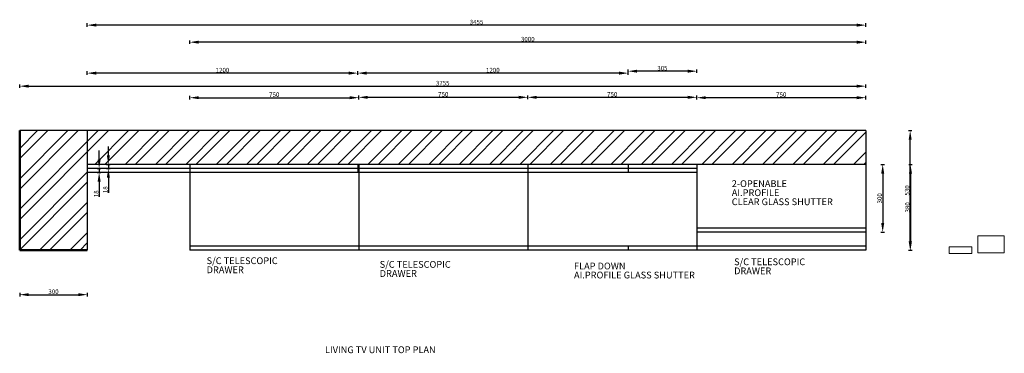
# Model space of a CAD drawing. Units: millimetres. Extents: x -4231 to 8464, y -424 to 4269.
# Tile 1 of 2: x -4231 to 139, y -424 to 1054. Entities that reach past the tile are written whole.
import ezdxf

# ---------------------------------------------------------------- set-up
doc = ezdxf.new("R2010")
doc.units = ezdxf.units.MM
for name, color, linetype, lineweight in [('A-ANNO-DIMS', 2, 'Continuous', 18), ('A-ANNO-IMAG', 7, 'Continuous', 18), ('A-ANNO-TEXT', 3, 'Continuous', 18), ('A-FURN', 30, 'Continuous', 25), ('A-WALL', 7, 'Continuous', 50), ('A-WALL-PATT', 8, 'Continuous', 13)]:
    doc.layers.add(name, color=color, linetype=linetype, lineweight=lineweight)
doc.styles.get("Standard").update_dxf_attribs({"font": 'arial.ttf', "height": 20})
doc.dimstyles.new('ISO-25', dxfattribs={"dimtxt": 40, "dimasz": 40, "dimexe": 8, "dimexo": 8, "dimtad": 1, "dimdec": 0, "dimtxsty": 'Standard', "dimcen": 2.5, "dimadec": 0, "dimazin": 0, "dimtfac": 1, "dimtdec": 0, "dimtmove": 0, "dimatfit": 3, "dimfxl": 8, "dimfxlon": 1, "dimarcsym": 0})
picture_1 = doc.add_image_def('image1.jpeg', size_in_pixel=(996, 302))
picture_2 = doc.add_image_def('image2.jpeg', size_in_pixel=(1062, 687))

# ---------------------------------------------------------------- blocks, each defined once
blk = doc.blocks.new('*D1')
at = {"layer": 'A-ANNO-DIMS', "color": 0, "lineweight": -2, "transparency": 16777216}
for p, q in [((-409.2, 412.6), (-393.2, 412.6)), ((-401.2, 372.6), (-401.2, 152.6)), ((-409.2, 112.6), (-393.2, 112.6))]:
    blk.add_line(p, q, dxfattribs=at)
at = {"layer": 'A-ANNO-DIMS', "color": 0, "transparency": 16777216}
for points in [[(-407.8, 372.6), (-394.5, 372.6), (-401.2, 412.6)], [(-407.8, 152.6), (-394.5, 152.6), (-401.2, 112.6)]]:
    blk.add_solid(points, dxfattribs=at)
at = {"layer": 'Defpoints', "color": 0, "transparency": 16777216}
for p in [(-476.3, 412.6), (-476.3, 112.6), (-401.2, 112.6)]:
    blk.add_point(p, dxfattribs=at)
at = {"layer": 'A-ANNO-DIMS', "color": 0, "transparency": 16777216, "insert": (-412, 262.6), "char_height": 20, "attachment_point": 5, "rotation": 90}
blk.add_mtext('300', dxfattribs=at)
blk = doc.blocks.new('*D2')
at = {"layer": 'A-ANNO-DIMS', "color": 0, "lineweight": -2, "transparency": 16777216}
for p, q in [((-285.9, 412.6), (-269.9, 412.6)), ((-277.9, 372.6), (-277.9, 72.6)), ((-285.9, 32.6), (-269.9, 32.6))]:
    blk.add_line(p, q, dxfattribs=at)
at = {"layer": 'A-ANNO-DIMS', "color": 0, "transparency": 16777216}
for points in [[(-284.6, 372.6), (-271.2, 372.6), (-277.9, 412.6)], [(-284.6, 72.6), (-271.2, 72.6), (-277.9, 32.6)]]:
    blk.add_solid(points, dxfattribs=at)
at = {"layer": 'Defpoints', "color": 0, "transparency": 16777216}
for p in [(-476.3, 412.6), (-476.3, 32.6), (-277.9, 32.6)]:
    blk.add_point(p, dxfattribs=at)
at = {"layer": 'A-ANNO-DIMS', "color": 0, "transparency": 16777216, "insert": (-288.8, 222.6), "char_height": 20, "attachment_point": 5, "rotation": 90}
blk.add_mtext('380', dxfattribs=at)
blk = doc.blocks.new('*D3')
at = {"layer": 'A-ANNO-DIMS', "color": 0, "lineweight": -2, "transparency": 16777216}
for p, q in [((-3931.3, 1022.1), (-3931.3, 1038.1)), ((-516.3, 1030.1), (-3891.3, 1030.1)), ((-476.3, 1022.1), (-476.3, 1038.1))]:
    blk.add_line(p, q, dxfattribs=at)
at = {"layer": 'A-ANNO-DIMS', "color": 0, "transparency": 16777216}
for points in [[(-3891.3, 1036.8), (-3891.3, 1023.5), (-3931.3, 1030.1)], [(-516.3, 1036.8), (-516.3, 1023.5), (-476.3, 1030.1)]]:
    blk.add_solid(points, dxfattribs=at)
at = {"layer": 'Defpoints', "color": 0, "transparency": 16777216}
for p in [(-3931.3, 1030.1), (-3931.3, 562.6), (-476.3, 562.6)]:
    blk.add_point(p, dxfattribs=at)
at = {"layer": 'A-ANNO-DIMS', "color": 0, "transparency": 16777216, "insert": (-2203.8, 1041), "char_height": 20, "attachment_point": 5}
blk.add_mtext('3455', dxfattribs=at)
blk = doc.blocks.new('*D4')
at = {"layer": 'A-ANNO-DIMS', "color": 0, "lineweight": -2, "transparency": 16777216}
for p, q in [((-1226.3, 700.5), (-1226.3, 716.5)), ((-516.3, 708.5), (-1186.3, 708.5)), ((-476.3, 700.5), (-476.3, 716.5))]:
    blk.add_line(p, q, dxfattribs=at)
at = {"layer": 'A-ANNO-DIMS', "color": 0, "transparency": 16777216}
for points in [[(-1186.3, 715.2), (-1186.3, 701.9), (-1226.3, 708.5)], [(-516.3, 715.2), (-516.3, 701.9), (-476.3, 708.5)]]:
    blk.add_solid(points, dxfattribs=at)
at = {"layer": 'Defpoints', "color": 0, "transparency": 16777216}
for p in [(-1226.3, 708.5), (-1226.3, 412.6), (-476.3, 412.6)]:
    blk.add_point(p, dxfattribs=at)
at = {"layer": 'A-ANNO-DIMS', "color": 0, "transparency": 16777216, "insert": (-851.3, 719.4), "char_height": 20, "attachment_point": 5}
blk.add_mtext('750', dxfattribs=at)
blk = doc.blocks.new('*D5')
at = {"layer": 'A-ANNO-DIMS', "color": 0, "lineweight": -2, "transparency": 16777216}
for p, q in [((-1976.3, 702.2), (-1976.3, 718.2)), ((-1936.3, 710.2), (-1266.3, 710.2)), ((-1226.3, 702.2), (-1226.3, 718.2))]:
    blk.add_line(p, q, dxfattribs=at)
at = {"layer": 'A-ANNO-DIMS', "color": 0, "transparency": 16777216}
for points in [[(-1936.3, 716.9), (-1936.3, 703.5), (-1976.3, 710.2)], [(-1266.3, 716.9), (-1266.3, 703.5), (-1226.3, 710.2)]]:
    blk.add_solid(points, dxfattribs=at)
at = {"layer": 'Defpoints', "color": 0, "transparency": 16777216}
for p in [(-1226.3, 710.2), (-1976.3, 412.6), (-1226.3, 412.6)]:
    blk.add_point(p, dxfattribs=at)
at = {"layer": 'A-ANNO-DIMS', "color": 0, "transparency": 16777216, "insert": (-1601.3, 721), "char_height": 20, "attachment_point": 5}
blk.add_mtext('750', dxfattribs=at)
blk = doc.blocks.new('*D6')
at = {"layer": 'A-ANNO-DIMS', "color": 0, "lineweight": -2, "transparency": 16777216}
for p, q in [((-2726.3, 702.2), (-2726.3, 718.2)), ((-2686.3, 710.2), (-2016.3, 710.2)), ((-1976.3, 702.2), (-1976.3, 718.2))]:
    blk.add_line(p, q, dxfattribs=at)
at = {"layer": 'A-ANNO-DIMS', "color": 0, "transparency": 16777216}
for points in [[(-2686.3, 716.9), (-2686.3, 703.5), (-2726.3, 710.2)], [(-2016.3, 716.9), (-2016.3, 703.5), (-1976.3, 710.2)]]:
    blk.add_solid(points, dxfattribs=at)
at = {"layer": 'Defpoints', "color": 0, "transparency": 16777216}
for p in [(-1976.3, 710.2), (-2726.3, 412.6), (-1976.3, 412.6)]:
    blk.add_point(p, dxfattribs=at)
at = {"layer": 'A-ANNO-DIMS', "color": 0, "transparency": 16777216, "insert": (-2351.3, 721), "char_height": 20, "attachment_point": 5}
blk.add_mtext('750', dxfattribs=at)
blk = doc.blocks.new('*D7')
at = {"layer": 'A-ANNO-DIMS', "color": 0, "lineweight": -2, "transparency": 16777216}
for p, q in [((-3476.3, 700.5), (-3476.3, 716.5)), ((-3436.3, 708.5), (-2766.3, 708.5)), ((-2726.3, 700.5), (-2726.3, 716.5))]:
    blk.add_line(p, q, dxfattribs=at)
at = {"layer": 'A-ANNO-DIMS', "color": 0, "transparency": 16777216}
for points in [[(-3436.3, 715.2), (-3436.3, 701.9), (-3476.3, 708.5)], [(-2766.3, 715.2), (-2766.3, 701.9), (-2726.3, 708.5)]]:
    blk.add_solid(points, dxfattribs=at)
at = {"layer": 'Defpoints', "color": 0, "transparency": 16777216}
for p in [(-2726.3, 708.5), (-3476.3, 412.6), (-2726.3, 412.6)]:
    blk.add_point(p, dxfattribs=at)
at = {"layer": 'A-ANNO-DIMS', "color": 0, "transparency": 16777216, "insert": (-3101.3, 719.4), "char_height": 20, "attachment_point": 5}
blk.add_mtext('750', dxfattribs=at)
blk = doc.blocks.new('*D8')
at = {"layer": 'A-ANNO-DIMS', "color": 0, "lineweight": -2, "transparency": 16777216}
for p, q in [((-3837.8, 452.6), (-3837.8, 492.6)), ((-3845.8, 412.6), (-3829.8, 412.6)), ((-3845.8, 394.6), (-3829.8, 394.6)), ((-3837.8, 412.6), (-3837.8, 394.6)), ((-3837.8, 354.6), (-3837.8, 286.6))]:
    blk.add_line(p, q, dxfattribs=at)
at = {"layer": 'A-ANNO-DIMS', "color": 0, "transparency": 16777216}
for points in [[(-3844.5, 452.6), (-3831.1, 452.6), (-3837.8, 412.6)], [(-3844.5, 354.6), (-3831.1, 354.6), (-3837.8, 394.6)]]:
    blk.add_solid(points, dxfattribs=at)
at = {"layer": 'Defpoints', "color": 0, "transparency": 16777216}
for p in [(-3931.3, 412.6), (-3931.3, 394.6), (-3837.8, 394.6)]:
    blk.add_point(p, dxfattribs=at)
at = {"layer": 'A-ANNO-DIMS', "color": 0, "transparency": 16777216, "insert": (-3848.6, 300.6), "char_height": 20, "attachment_point": 5, "rotation": 90}
blk.add_mtext('18', dxfattribs=at)
blk = doc.blocks.new('*D9')
at = {"layer": 'A-ANNO-DIMS', "color": 0, "lineweight": -2, "transparency": 16777216}
for p, q in [((-3878.7, 434.6), (-3878.7, 474.6)), ((-3886.7, 394.6), (-3870.7, 394.6)), ((-3878.7, 394.6), (-3878.7, 376.6)), ((-3886.7, 376.6), (-3870.7, 376.6)), ((-3878.7, 336.6), (-3878.7, 268.6))]:
    blk.add_line(p, q, dxfattribs=at)
at = {"layer": 'A-ANNO-DIMS', "color": 0, "transparency": 16777216}
for points in [[(-3885.4, 434.6), (-3872, 434.6), (-3878.7, 394.6)], [(-3885.4, 336.6), (-3872, 336.6), (-3878.7, 376.6)]]:
    blk.add_solid(points, dxfattribs=at)
at = {"layer": 'Defpoints', "color": 0, "transparency": 16777216}
for p in [(-3931.3, 394.6), (-3924.2, 376.6), (-3878.7, 376.6)]:
    blk.add_point(p, dxfattribs=at)
at = {"layer": 'A-ANNO-DIMS', "color": 0, "transparency": 16777216, "insert": (-3889.5, 282.6), "char_height": 20, "attachment_point": 5, "rotation": 90}
blk.add_mtext('18', dxfattribs=at)
blk = doc.blocks.new('*D10')
at = {"layer": 'A-ANNO-DIMS', "color": 0, "lineweight": -2, "transparency": 16777216}
for p, q in [((-3931.3, 809.4), (-3931.3, 825.4)), ((-2771.3, 817.4), (-3891.3, 817.4)), ((-2731.3, 809.4), (-2731.3, 825.4))]:
    blk.add_line(p, q, dxfattribs=at)
at = {"layer": 'A-ANNO-DIMS', "color": 0, "transparency": 16777216}
for points in [[(-3891.3, 824.1), (-3891.3, 810.7), (-3931.3, 817.4)], [(-2771.3, 824.1), (-2771.3, 810.7), (-2731.3, 817.4)]]:
    blk.add_solid(points, dxfattribs=at)
at = {"layer": 'Defpoints', "color": 0, "transparency": 16777216}
for p in [(-3931.3, 817.4), (-3931.3, 376.6), (-2731.3, 376.6)]:
    blk.add_point(p, dxfattribs=at)
at = {"layer": 'A-ANNO-DIMS', "color": 0, "transparency": 16777216, "insert": (-3331.3, 828.2), "char_height": 20, "attachment_point": 5}
blk.add_mtext('1200', dxfattribs=at)
blk = doc.blocks.new('*D11')
at = {"layer": 'A-ANNO-DIMS', "color": 0, "lineweight": -2, "transparency": 16777216}
for p, q in [((-1531.3, 818), (-1531.3, 834)), ((-1226.3, 818), (-1226.3, 834)), ((-1266.3, 826), (-1491.3, 826))]:
    blk.add_line(p, q, dxfattribs=at)
at = {"layer": 'A-ANNO-DIMS', "color": 0, "transparency": 16777216}
for points in [[(-1491.3, 832.6), (-1491.3, 819.3), (-1531.3, 826)], [(-1266.3, 832.6), (-1266.3, 819.3), (-1226.3, 826)]]:
    blk.add_solid(points, dxfattribs=at)
at = {"layer": 'Defpoints', "color": 0, "transparency": 16777216}
for p in [(-1531.3, 826), (-1531.3, 412.6), (-1226.3, 412.6)]:
    blk.add_point(p, dxfattribs=at)
at = {"layer": 'A-ANNO-DIMS', "color": 0, "transparency": 16777216, "insert": (-1378.8, 836.8), "char_height": 20, "attachment_point": 5}
blk.add_mtext('305', dxfattribs=at)
blk = doc.blocks.new('*D12')
at = {"layer": 'A-ANNO-DIMS', "color": 0, "lineweight": -2, "transparency": 16777216}
for p, q in [((-2731.3, 809.4), (-2731.3, 825.4)), ((-1571.3, 817.4), (-2691.3, 817.4)), ((-1531.3, 809.4), (-1531.3, 825.4))]:
    blk.add_line(p, q, dxfattribs=at)
at = {"layer": 'A-ANNO-DIMS', "color": 0, "transparency": 16777216}
for points in [[(-2691.3, 824.1), (-2691.3, 810.7), (-2731.3, 817.4)], [(-1571.3, 824.1), (-1571.3, 810.7), (-1531.3, 817.4)]]:
    blk.add_solid(points, dxfattribs=at)
at = {"layer": 'Defpoints', "color": 0, "transparency": 16777216}
for p in [(-2731.3, 817.4), (-2731.3, 412.6), (-1531.3, 412.6)]:
    blk.add_point(p, dxfattribs=at)
at = {"layer": 'A-ANNO-DIMS', "color": 0, "transparency": 16777216, "insert": (-2131.3, 828.2), "char_height": 20, "attachment_point": 5}
blk.add_mtext('1200', dxfattribs=at)
blk = doc.blocks.new('*D13')
at = {"layer": 'A-ANNO-DIMS', "color": 0, "lineweight": -2, "transparency": 16777216}
for p, q in [((-3476.3, 946.6), (-3476.3, 962.6)), ((-476.3, 946.6), (-476.3, 962.6)), ((-516.3, 954.6), (-3436.3, 954.6))]:
    blk.add_line(p, q, dxfattribs=at)
at = {"layer": 'A-ANNO-DIMS', "color": 0, "transparency": 16777216}
for points in [[(-3436.3, 961.3), (-3436.3, 947.9), (-3476.3, 954.6)], [(-516.3, 961.3), (-516.3, 947.9), (-476.3, 954.6)]]:
    blk.add_solid(points, dxfattribs=at)
at = {"layer": 'Defpoints', "color": 0, "transparency": 16777216}
for p in [(-3476.3, 954.6), (-3476.3, 412.6), (-476.3, 412.6)]:
    blk.add_point(p, dxfattribs=at)
at = {"layer": 'A-ANNO-DIMS', "color": 0, "transparency": 16777216, "insert": (-1976.3, 965.4), "char_height": 20, "attachment_point": 5}
blk.add_mtext('3000', dxfattribs=at)
blk = doc.blocks.new('*D31')
at = {"layer": 'A-ANNO-DIMS', "color": 0, "lineweight": -2, "transparency": 16777216}
for p, q in [((-287.3, 562.6), (-271.3, 562.6)), ((-279.3, 72.6), (-279.3, 522.6)), ((-287.3, 32.6), (-271.3, 32.6))]:
    blk.add_line(p, q, dxfattribs=at)
at = {"layer": 'A-ANNO-DIMS', "color": 0, "transparency": 16777216}
for points in [[(-285.9, 522.6), (-272.6, 522.6), (-279.3, 562.6)], [(-285.9, 72.6), (-272.6, 72.6), (-279.3, 32.6)]]:
    blk.add_solid(points, dxfattribs=at)
at = {"layer": 'Defpoints', "color": 0, "transparency": 16777216}
for p in [(-476.3, 562.6), (-279.3, 562.6), (-476.3, 32.6)]:
    blk.add_point(p, dxfattribs=at)
at = {"layer": 'A-ANNO-DIMS', "color": 0, "transparency": 16777216, "insert": (-290.1, 297.6), "char_height": 20, "attachment_point": 5, "rotation": 90}
blk.add_mtext('530', dxfattribs=at)
blk = doc.blocks.new('*D32')
at = {"layer": 'A-ANNO-DIMS', "color": 0, "lineweight": -2, "transparency": 16777216}
for p, q in [((-4231.3, 751.6), (-4231.3, 767.6)), ((-4191.3, 759.6), (-516.3, 759.6)), ((-476.3, 751.6), (-476.3, 767.6))]:
    blk.add_line(p, q, dxfattribs=at)
at = {"layer": 'A-ANNO-DIMS', "color": 0, "transparency": 16777216}
for points in [[(-4191.3, 766.3), (-4191.3, 753), (-4231.3, 759.6)], [(-516.3, 766.3), (-516.3, 753), (-476.3, 759.6)]]:
    blk.add_solid(points, dxfattribs=at)
at = {"layer": 'Defpoints', "color": 0, "transparency": 16777216}
for p in [(-476.3, 759.6), (-4231.3, 562.6), (-476.3, 562.6)]:
    blk.add_point(p, dxfattribs=at)
at = {"layer": 'A-ANNO-DIMS', "color": 0, "transparency": 16777216, "insert": (-2353.8, 770.5), "char_height": 20, "attachment_point": 5}
blk.add_mtext('3755', dxfattribs=at)
blk = doc.blocks.new('*D33')
at = {"layer": 'A-ANNO-DIMS', "color": 0, "lineweight": -2, "transparency": 16777216}
for p, q in [((-4231.3, -156.4), (-4231.3, -172.4)), ((-4191.3, -164.4), (-3971.3, -164.4)), ((-3931.3, -156.4), (-3931.3, -172.4))]:
    blk.add_line(p, q, dxfattribs=at)
at = {"layer": 'A-ANNO-DIMS', "color": 0, "transparency": 16777216}
for points in [[(-4191.3, -157.7), (-4191.3, -171), (-4231.3, -164.4)], [(-3971.3, -157.7), (-3971.3, -171), (-3931.3, -164.4)]]:
    blk.add_solid(points, dxfattribs=at)
at = {"layer": 'Defpoints', "color": 0, "transparency": 16777216}
for p in [(-4231.3, 32.6), (-3931.3, 32.6), (-3931.3, -164.4)]:
    blk.add_point(p, dxfattribs=at)
at = {"layer": 'A-ANNO-DIMS', "color": 0, "transparency": 16777216, "insert": (-4081.3, -153.5), "char_height": 20, "attachment_point": 5}
blk.add_mtext('300', dxfattribs=at)

msp = doc.modelspace()

# ---------------------------------------------------------------- hatches: boundary and pattern name
at = {"layer": 'A-WALL-PATT'}
h = msp.add_hatch(dxfattribs=at)
h.set_pattern_fill('ANSI32', color=256, scale=10)
h.paths.add_polyline_path([(-476.28, 562.64), (-3931.28, 562.64), (-3931.28, 412.64), (-476.28, 412.64)])
h.paths.add_polyline_path([(-3931.28, 562.64), (-4231.28, 562.64), (-4231.28, 32.64), (-3931.28, 32.64)])

# ---------------------------------------------------------------- linework, layer by layer
at = {"layer": 'A-FURN'}
for p, q in [((-476.28, 562.64), (-4231.28, 562.64)), ((-3931.28, 562.64), (-3931.28, 32.64)), ((-476.28, 562.64), (-476.28, 32.64)), ((-476.28, 412.64), (-3931.28, 412.64)), ((-1226.28, 394.64), (-3931.28, 394.64)), ((-3476.28, 412.64), (-3476.28, 32.64)), ((-2731.28, 412.64), (-2731.28, 376.64)), ((-2726.28, 412.64), (-2726.28, 32.64)), ((-1976.28, 412.64), (-1976.28, 32.64)), ((-1531.28, 412.64), (-1531.28, 376.64)), ((-1226.28, 412.64), (-1226.28, 32.64)), ((-1226.28, 376.64), (-3931.28, 376.64)), ((-476.28, 130.64), (-1226.28, 130.64)), ((-476.28, 112.64), (-1226.28, 112.64)), ((-476.28, 50.64), (-3476.28, 50.64)), ((-1531.28, 50.64), (-1531.28, 32.64)), ((-1226.28, 32.64), (-3476.28, 32.64)), ((-476.28, 32.64), (-1226.28, 32.64))]:
    msp.add_line(p, q, dxfattribs=at)
at = {"layer": 'A-WALL'}
for p, q in [((-4231.28, 32.64), (-4231.28, 562.64)), ((-3931.28, 32.64), (-4231.28, 32.64))]:
    msp.add_line(p, q, dxfattribs=at)

# ---------------------------------------------------------------- texts
at = {"layer": 'A-ANNO-TEXT'}
for s, p in [('2-OPENABLE', (-1071.08, 312.63)), ('AI.PROFILE', (-1071.08, 272.47)), ('CLEAR GLASS SHUTTER', (-1071.08, 232.31)), ('S/C TELESCOPIC ', (-3401.74, -28.95)), ('DRAWER', (-3401.74, -69.11)), ('S/C TELESCOPIC', (-2633.61, -45.21)), ('FLAP DOWN', (-1771.23, -52.37)), ('S/C TELESCOPIC', (-1060.69, -33.74)), ('DRAWER', (-2633.61, -85.37)), ('AI.PROFILE GLASS SHUTTER', (-1771.23, -92.53)), ('DRAWER', (-1060.69, -73.9)), ('LIVING TV UNIT TOP PLAN', (-2876.22, -423.56))]:
    msp.add_text(s, height=30, dxfattribs=at).set_placement(p)

# ---------------------------------------------------------------- dimensions: what is measured, and where the dimension line sits
at = {"layer": 'A-ANNO-DIMS'}
for base, p1, p2, override, picture, middle in [((-3931.28, 1030.14), (-476.28, 562.64), (-3931.28, 562.64), {"dimclrd": 0, "dimclre": 0, "dimclrt": 0}, '*D3', (-2203.78, 1040.98)), ((-3476.28, 954.59), (-476.28, 412.64), (-3476.28, 412.64), {"dimclrd": 0, "dimclre": 0, "dimclrt": 0}, '*D13', (-1976.28, 965.44)), ((-3931.28, 817.39), (-2731.28, 376.64), (-3931.28, 376.64), {"dimclrd": 0, "dimclre": 0, "dimclrt": 0}, '*D10', (-3331.28, 828.22)), ((-2731.28, 817.39), (-1531.28, 412.64), (-2731.28, 412.64), {"dimclrd": 0, "dimclre": 0, "dimclrt": 0}, '*D12', (-2131.28, 828.22)), ((-1531.28, 825.96), (-1226.28, 412.64), (-1531.28, 412.64), {"dimclrd": 0, "dimclre": 0, "dimclrt": 0}, '*D11', (-1378.78, 836.8)), ((-476.28, 759.64), (-4231.28, 562.64), (-476.28, 562.64), {"dimdec": 0, "dimlfac": 1, "dimrnd": 0, "dimzin": 0, "dimdsep": 46, "dimlunit": 2}, '*D32', (-2353.78, 770.48)), ((-2726.28, 708.54), (-3476.28, 412.64), (-2726.28, 412.64), {"dimclrd": 0, "dimclre": 0, "dimclrt": 0}, '*D7', (-3101.28, 719.38)), ((-1976.28, 710.21), (-2726.28, 412.64), (-1976.28, 412.64), {"dimclrd": 0, "dimclre": 0, "dimclrt": 0}, '*D6', (-2351.28, 721.05)), ((-1226.28, 710.21), (-1976.28, 412.64), (-1226.28, 412.64), {"dimclrd": 0, "dimclre": 0, "dimclrt": 0}, '*D5', (-1601.28, 721.05)), ((-1226.28, 708.54), (-476.28, 412.64), (-1226.28, 412.64), {"dimclrd": 0, "dimclre": 0, "dimclrt": 0}, '*D4', (-851.28, 719.38)), ((-3931.28, -164.36), (-4231.28, 32.64), (-3931.28, 32.64), {"dimdec": 0, "dimlfac": 1, "dimrnd": 0, "dimzin": 0, "dimdsep": 46, "dimlunit": 2}, '*D33', (-4081.28, -153.52))]:
    dim = msp.add_linear_dim(base=base, p1=p1, p2=p2, dimstyle='ISO-25', override=override, dxfattribs=at)
    dim.commit()
    dim.dimension.update_dxf_attribs({"geometry": picture, "text_midpoint": middle})
for base, p1, p2, override, picture, middle in [((-279.28, 562.64), (-476.28, 32.64), (-476.28, 562.64), {"dimdec": 0, "dimlfac": 1, "dimrnd": 0, "dimzin": 0, "dimdsep": 46, "dimlunit": 2}, '*D31', (-290.12, 297.64)), ((-3837.79, 394.64), (-3931.28, 412.64), (-3931.28, 394.64), {"dimclrd": 0, "dimclre": 0, "dimclrt": 0}, '*D8', (-3848.63, 300.61)), ((-3878.69, 376.64), (-3931.28, 394.64), (-3924.16, 376.64), {"dimclrd": 0, "dimclre": 0, "dimclrt": 0}, '*D9', (-3889.53, 282.61)), ((-401.17, 112.64), (-476.28, 412.64), (-476.28, 112.64), {"dimclrd": 0, "dimclre": 0, "dimclrt": 0}, '*D1', (-412.01, 262.64)), ((-277.91, 32.64), (-476.28, 412.64), (-476.28, 32.64), {"dimclrd": 0, "dimclre": 0, "dimclrt": 0}, '*D2', (-288.75, 222.64))]:
    dim = msp.add_linear_dim(base=base, p1=p1, p2=p2, angle=90, dimstyle='ISO-25', override=override, dxfattribs=at)
    dim.commit()
    dim.dimension.update_dxf_attribs({"geometry": picture, "text_midpoint": middle})

# ---------------------------------------------------------------- pictures from other files: only their frames are drawn
at = {"layer": 'A-ANNO-IMAG'}
image = msp.add_image(picture_2, insert=(21.16, 20.67), size_in_units=(117.4, 75.94), dxfattribs=at)
image.dxf.flags = 7
image = msp.add_image(picture_1, insert=(-106.33, 17.4), size_in_units=(100.68, 30.53), dxfattribs=at)
image.dxf.flags = 7

doc.saveas('drawing.dxf')
